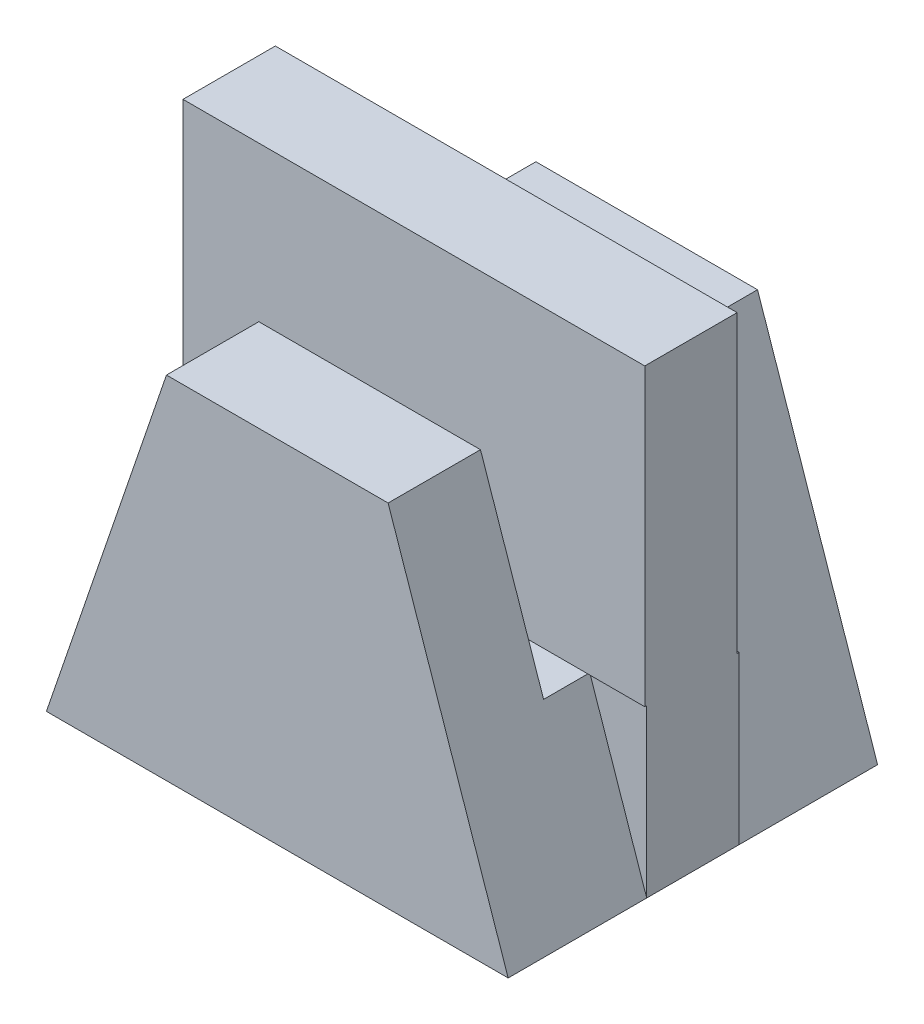
ISO-10303-21;
HEADER;
FILE_DESCRIPTION(('STEP AP214'),'2;1');
FILE_NAME('part.step','',(''),(''),'','','');
FILE_SCHEMA(('AUTOMOTIVE_DESIGN { 1 0 10303 214 1 1 1 1 }'));
ENDSEC;
DATA;
#1=APPLICATION_CONTEXT('core data for automotive mechanical design processes');
#2=APPLICATION_PROTOCOL_DEFINITION('international standard','automotive_design',2000,#1);
#3=PRODUCT_CONTEXT('',#1,'mechanical');
#4=PRODUCT('Part','Part','',(#3));
#5=PRODUCT_RELATED_PRODUCT_CATEGORY('part','',(#4));
#6=PRODUCT_DEFINITION_FORMATION('','',#4);
#7=PRODUCT_DEFINITION_CONTEXT('part definition',#1,'design');
#8=PRODUCT_DEFINITION('design','',#6,#7);
#9=PRODUCT_DEFINITION_SHAPE('','',#8);
#10=(LENGTH_UNIT() NAMED_UNIT(*) SI_UNIT(.MILLI.,.METRE.));
#11=(NAMED_UNIT(*) PLANE_ANGLE_UNIT() SI_UNIT($,.RADIAN.));
#12=(NAMED_UNIT(*) SI_UNIT($,.STERADIAN.) SOLID_ANGLE_UNIT());
#13=UNCERTAINTY_MEASURE_WITH_UNIT(LENGTH_MEASURE(1.E-05),#10,'distance_accuracy_value','');
#14=(GEOMETRIC_REPRESENTATION_CONTEXT(3) GLOBAL_UNCERTAINTY_ASSIGNED_CONTEXT((#13)) GLOBAL_UNIT_ASSIGNED_CONTEXT((#10,
#11,#12)) REPRESENTATION_CONTEXT('',''));
#15=CARTESIAN_POINT('',(0.,0.,0.));
#16=DIRECTION('',(0.,0.,1.));
#17=DIRECTION('',(1.,0.,0.));
#18=AXIS2_PLACEMENT_3D('',#15,#16,#17);
#19=CARTESIAN_POINT('',(25.,0.,40.));
#20=DIRECTION('',(1.,0.,0.));
#21=DIRECTION('',(0.,1.,0.));
#22=AXIS2_PLACEMENT_3D('',#19,#20,#21);
#23=PLANE('',#22);
#24=DIRECTION('',(0.,0.,1.));
#25=VECTOR('',#24,1.);
#26=CARTESIAN_POINT('',(25.,-6.95880702065631,25.));
#27=LINE('',#26,#25);
#28=CARTESIAN_POINT('',(25.,-6.95880702065631,25.));
#29=VERTEX_POINT('',#28);
#30=CARTESIAN_POINT('',(25.,-6.95880702065631,25.211069260478));
#31=VERTEX_POINT('',#30);
#32=EDGE_CURVE('E200',#29,#31,#27,.T.);
#33=ORIENTED_EDGE('',*,*,#32,.F.);
#34=DIRECTION('',(0.,1.,0.));
#35=VECTOR('',#34,1.);
#36=CARTESIAN_POINT('',(25.,-25.,25.));
#37=LINE('',#36,#35);
#38=CARTESIAN_POINT('',(25.,-25.,25.));
#39=VERTEX_POINT('',#38);
#40=EDGE_CURVE('E189',#39,#29,#37,.T.);
#41=ORIENTED_EDGE('',*,*,#40,.F.);
#42=DIRECTION('',(0.,0.,-1.));
#43=VECTOR('',#42,1.);
#44=CARTESIAN_POINT('',(25.,-25.,40.));
#45=LINE('',#44,#43);
#46=CARTESIAN_POINT('',(25.,-25.,15.));
#47=VERTEX_POINT('',#46);
#48=EDGE_CURVE('E183',#39,#47,#45,.T.);
#49=ORIENTED_EDGE('',*,*,#48,.T.);
#50=DIRECTION('',(0.,-1.,0.));
#51=VECTOR('',#50,1.);
#52=CARTESIAN_POINT('',(25.,-6.9588070206563,15.));
#53=LINE('',#52,#51);
#54=CARTESIAN_POINT('',(25.,-6.9588070206563,15.));
#55=VERTEX_POINT('',#54);
#56=EDGE_CURVE('E318',#55,#47,#53,.T.);
#57=ORIENTED_EDGE('',*,*,#56,.F.);
#58=DIRECTION('',(0.,0.,1.));
#59=VECTOR('',#58,1.);
#60=CARTESIAN_POINT('',(25.,-6.9588070206563,0.));
#61=LINE('',#60,#59);
#62=CARTESIAN_POINT('',(25.,-6.9588070206563,15.211069260478));
#63=VERTEX_POINT('',#62);
#64=EDGE_CURVE('E231',#55,#63,#61,.T.);
#65=ORIENTED_EDGE('',*,*,#64,.T.);
#66=DIRECTION('',(0.,1.,0.));
#67=VECTOR('',#66,1.);
#68=CARTESIAN_POINT('',(25.,0.,15.211069260478));
#69=LINE('',#68,#67);
#70=CARTESIAN_POINT('',(25.,25.,15.211069260478));
#71=VERTEX_POINT('',#70);
#72=EDGE_CURVE('E236',#63,#71,#69,.T.);
#73=ORIENTED_EDGE('',*,*,#72,.T.);
#74=DIRECTION('',(0.,0.,-1.));
#75=VECTOR('',#74,1.);
#76=CARTESIAN_POINT('',(25.,25.,40.));
#77=LINE('',#76,#75);
#78=CARTESIAN_POINT('',(25.,25.,25.211069260478));
#79=VERTEX_POINT('',#78);
#80=EDGE_CURVE('E202',#79,#71,#77,.T.);
#81=ORIENTED_EDGE('',*,*,#80,.F.);
#82=DIRECTION('',(0.,-1.,0.));
#83=VECTOR('',#82,1.);
#84=CARTESIAN_POINT('',(25.,0.,25.211069260478));
#85=LINE('',#84,#83);
#86=EDGE_CURVE('E235',#79,#31,#85,.T.);
#87=ORIENTED_EDGE('',*,*,#86,.T.);
#88=EDGE_LOOP('',(#33,#41,#49,#57,#65,#73,#81,#87));
#89=FACE_BOUND('',#88,.T.);
#90=ADVANCED_FACE('F43',(#89),#23,.T.);
#91=CARTESIAN_POINT('',(-25.,0.,40.));
#92=DIRECTION('',(1.,0.,0.));
#93=DIRECTION('',(0.,1.,0.));
#94=AXIS2_PLACEMENT_3D('',#91,#92,#93);
#95=PLANE('',#94);
#96=DIRECTION('',(0.,0.,1.));
#97=VECTOR('',#96,1.);
#98=CARTESIAN_POINT('',(-25.,-6.95880702065631,0.));
#99=LINE('',#98,#97);
#100=CARTESIAN_POINT('',(-25.,-6.95880702065631,15.));
#101=VERTEX_POINT('',#100);
#102=CARTESIAN_POINT('',(-25.,-6.95880702065631,15.211069260478));
#103=VERTEX_POINT('',#102);
#104=EDGE_CURVE('E221',#101,#103,#99,.T.);
#105=ORIENTED_EDGE('',*,*,#104,.F.);
#106=DIRECTION('',(0.,1.,0.));
#107=VECTOR('',#106,1.);
#108=CARTESIAN_POINT('',(-25.,-25.,15.));
#109=LINE('',#108,#107);
#110=CARTESIAN_POINT('',(-25.,-25.,15.));
#111=VERTEX_POINT('',#110);
#112=EDGE_CURVE('E308',#111,#101,#109,.T.);
#113=ORIENTED_EDGE('',*,*,#112,.F.);
#114=DIRECTION('',(0.,0.,-1.));
#115=VECTOR('',#114,1.);
#116=CARTESIAN_POINT('',(-25.,-25.,40.));
#117=LINE('',#116,#115);
#118=CARTESIAN_POINT('',(-25.,-25.,25.));
#119=VERTEX_POINT('',#118);
#120=EDGE_CURVE('E212',#119,#111,#117,.T.);
#121=ORIENTED_EDGE('',*,*,#120,.F.);
#122=DIRECTION('',(0.,-1.,0.));
#123=VECTOR('',#122,1.);
#124=CARTESIAN_POINT('',(-25.,-25.,25.));
#125=LINE('',#124,#123);
#126=CARTESIAN_POINT('',(-25.,-6.95880702065632,25.));
#127=VERTEX_POINT('',#126);
#128=EDGE_CURVE('E295',#127,#119,#125,.T.);
#129=ORIENTED_EDGE('',*,*,#128,.F.);
#130=DIRECTION('',(0.,0.,1.));
#131=VECTOR('',#130,1.);
#132=CARTESIAN_POINT('',(-25.,-6.95880702065632,25.));
#133=LINE('',#132,#131);
#134=CARTESIAN_POINT('',(-25.,-6.95880702065632,25.211069260478));
#135=VERTEX_POINT('',#134);
#136=EDGE_CURVE('E286',#127,#135,#133,.T.);
#137=ORIENTED_EDGE('',*,*,#136,.T.);
#138=DIRECTION('',(0.,-1.,0.));
#139=VECTOR('',#138,1.);
#140=CARTESIAN_POINT('',(-25.,0.,25.211069260478));
#141=LINE('',#140,#139);
#142=CARTESIAN_POINT('',(-25.,25.,25.211069260478));
#143=VERTEX_POINT('',#142);
#144=EDGE_CURVE('E246',#143,#135,#141,.T.);
#145=ORIENTED_EDGE('',*,*,#144,.F.);
#146=DIRECTION('',(0.,0.,-1.));
#147=VECTOR('',#146,1.);
#148=CARTESIAN_POINT('',(-25.,25.,40.));
#149=LINE('',#148,#147);
#150=CARTESIAN_POINT('',(-25.,25.,15.211069260478));
#151=VERTEX_POINT('',#150);
#152=EDGE_CURVE('E203',#143,#151,#149,.T.);
#153=ORIENTED_EDGE('',*,*,#152,.T.);
#154=DIRECTION('',(0.,1.,0.));
#155=VECTOR('',#154,1.);
#156=CARTESIAN_POINT('',(-25.,0.,15.211069260478));
#157=LINE('',#156,#155);
#158=EDGE_CURVE('E232',#103,#151,#157,.T.);
#159=ORIENTED_EDGE('',*,*,#158,.F.);
#160=EDGE_LOOP('',(#105,#113,#121,#129,#137,#145,#153,#159));
#161=FACE_BOUND('',#160,.T.);
#162=ADVANCED_FACE('F341',(#161),#95,.F.);
#163=CARTESIAN_POINT('',(0.,25.,40.));
#164=DIRECTION('',(0.,1.,0.));
#165=DIRECTION('',(-1.,0.,0.));
#166=AXIS2_PLACEMENT_3D('',#163,#164,#165);
#167=PLANE('',#166);
#168=ORIENTED_EDGE('',*,*,#152,.F.);
#169=DIRECTION('',(1.,0.,0.));
#170=VECTOR('',#169,1.);
#171=CARTESIAN_POINT('',(-25.,25.,25.211069260478));
#172=LINE('',#171,#170);
#173=EDGE_CURVE('E254',#143,#79,#172,.T.);
#174=ORIENTED_EDGE('',*,*,#173,.T.);
#175=ORIENTED_EDGE('',*,*,#80,.T.);
#176=DIRECTION('',(1.,0.,0.));
#177=VECTOR('',#176,1.);
#178=CARTESIAN_POINT('',(-25.,25.,15.211069260478));
#179=LINE('',#178,#177);
#180=EDGE_CURVE('E223',#151,#71,#179,.T.);
#181=ORIENTED_EDGE('',*,*,#180,.F.);
#182=EDGE_LOOP('',(#168,#174,#175,#181));
#183=FACE_BOUND('',#182,.T.);
#184=ADVANCED_FACE('F395',(#183),#167,.T.);
#185=CARTESIAN_POINT('',(0.,0.,40.));
#186=DIRECTION('',(0.,0.,1.));
#187=DIRECTION('',(1.,0.,0.));
#188=AXIS2_PLACEMENT_3D('',#185,#186,#187);
#189=PLANE('',#188);
#190=DIRECTION('',(0.323373843640664,-0.94627129156974,0.));
#191=VECTOR('',#190,1.);
#192=CARTESIAN_POINT('',(12.,13.0411929793437,40.));
#193=LINE('',#192,#191);
#194=CARTESIAN_POINT('',(12.,13.0411929793437,40.));
#195=VERTEX_POINT('',#194);
#196=CARTESIAN_POINT('',(25.,-25.,40.));
#197=VERTEX_POINT('',#196);
#198=EDGE_CURVE('E177',#195,#197,#193,.T.);
#199=ORIENTED_EDGE('',*,*,#198,.F.);
#200=DIRECTION('',(1.,0.,0.));
#201=VECTOR('',#200,1.);
#202=CARTESIAN_POINT('',(-25.,13.0411929793437,40.));
#203=LINE('',#202,#201);
#204=CARTESIAN_POINT('',(-12.,13.0411929793437,40.));
#205=VERTEX_POINT('',#204);
#206=EDGE_CURVE('E213',#205,#195,#203,.T.);
#207=ORIENTED_EDGE('',*,*,#206,.F.);
#208=DIRECTION('',(0.323373843640664,0.94627129156974,0.));
#209=VECTOR('',#208,1.);
#210=CARTESIAN_POINT('',(-25.,-25.,40.));
#211=LINE('',#210,#209);
#212=CARTESIAN_POINT('',(-25.,-25.,40.));
#213=VERTEX_POINT('',#212);
#214=EDGE_CURVE('E284',#213,#205,#211,.T.);
#215=ORIENTED_EDGE('',*,*,#214,.F.);
#216=DIRECTION('',(1.,0.,0.));
#217=VECTOR('',#216,1.);
#218=CARTESIAN_POINT('',(0.,-25.,40.));
#219=LINE('',#218,#217);
#220=EDGE_CURVE('E211',#213,#197,#219,.T.);
#221=ORIENTED_EDGE('',*,*,#220,.T.);
#222=EDGE_LOOP('',(#199,#207,#215,#221));
#223=FACE_BOUND('',#222,.T.);
#224=ADVANCED_FACE('F365',(#223),#189,.T.);
#225=CARTESIAN_POINT('',(0.,0.,0.));
#226=DIRECTION('',(0.,0.,1.));
#227=DIRECTION('',(1.,0.,0.));
#228=AXIS2_PLACEMENT_3D('',#225,#226,#227);
#229=PLANE('',#228);
#230=DIRECTION('',(1.,0.,0.));
#231=VECTOR('',#230,1.);
#232=CARTESIAN_POINT('',(0.,-25.,0.));
#233=LINE('',#232,#231);
#234=CARTESIAN_POINT('',(-25.,-25.,0.));
#235=VERTEX_POINT('',#234);
#236=CARTESIAN_POINT('',(25.,-25.,0.));
#237=VERTEX_POINT('',#236);
#238=EDGE_CURVE('E215',#235,#237,#233,.T.);
#239=ORIENTED_EDGE('',*,*,#238,.F.);
#240=DIRECTION('',(-0.323373843640664,-0.94627129156974,0.));
#241=VECTOR('',#240,1.);
#242=CARTESIAN_POINT('',(-12.,13.0411929793437,0.));
#243=LINE('',#242,#241);
#244=CARTESIAN_POINT('',(-12.,13.0411929793437,0.));
#245=VERTEX_POINT('',#244);
#246=EDGE_CURVE('E270',#245,#235,#243,.T.);
#247=ORIENTED_EDGE('',*,*,#246,.F.);
#248=DIRECTION('',(1.,0.,0.));
#249=VECTOR('',#248,1.);
#250=CARTESIAN_POINT('',(-25.,13.0411929793437,0.));
#251=LINE('',#250,#249);
#252=CARTESIAN_POINT('',(12.,13.0411929793437,0.));
#253=VERTEX_POINT('',#252);
#254=EDGE_CURVE('E217',#245,#253,#251,.T.);
#255=ORIENTED_EDGE('',*,*,#254,.T.);
#256=DIRECTION('',(-0.323373843640664,0.94627129156974,0.));
#257=VECTOR('',#256,1.);
#258=CARTESIAN_POINT('',(12.,13.0411929793437,0.));
#259=LINE('',#258,#257);
#260=EDGE_CURVE('E271',#237,#253,#259,.T.);
#261=ORIENTED_EDGE('',*,*,#260,.F.);
#262=EDGE_LOOP('',(#239,#247,#255,#261));
#263=FACE_BOUND('',#262,.T.);
#264=ADVANCED_FACE('F368',(#263),#229,.F.);
#265=CARTESIAN_POINT('',(0.,-25.,40.));
#266=DIRECTION('',(0.,1.,0.));
#267=DIRECTION('',(0.,0.,1.));
#268=AXIS2_PLACEMENT_3D('',#265,#266,#267);
#269=PLANE('',#268);
#270=ORIENTED_EDGE('',*,*,#238,.T.);
#271=DIRECTION('',(0.,0.,-1.));
#272=VECTOR('',#271,1.);
#273=CARTESIAN_POINT('',(25.,-25.,10.));
#274=LINE('',#273,#272);
#275=EDGE_CURVE('E197',#47,#237,#274,.T.);
#276=ORIENTED_EDGE('',*,*,#275,.F.);
#277=ORIENTED_EDGE('',*,*,#48,.F.);
#278=EDGE_CURVE('E51',#197,#39,#45,.T.);
#279=ORIENTED_EDGE('',*,*,#278,.F.);
#280=ORIENTED_EDGE('',*,*,#220,.F.);
#281=EDGE_CURVE('E209',#213,#119,#117,.T.);
#282=ORIENTED_EDGE('',*,*,#281,.T.);
#283=ORIENTED_EDGE('',*,*,#120,.T.);
#284=DIRECTION('',(0.,0.,-1.));
#285=VECTOR('',#284,1.);
#286=CARTESIAN_POINT('',(-25.,-25.,10.));
#287=LINE('',#286,#285);
#288=EDGE_CURVE('E237',#111,#235,#287,.T.);
#289=ORIENTED_EDGE('',*,*,#288,.T.);
#290=EDGE_LOOP('',(#270,#276,#277,#279,#280,#282,#283,#289));
#291=FACE_BOUND('',#290,.T.);
#292=ADVANCED_FACE('F44',(#291),#269,.F.);
#293=CARTESIAN_POINT('',(-25.,0.,10.));
#294=DIRECTION('',(0.,0.,1.));
#295=DIRECTION('',(0.,-1.,0.));
#296=AXIS2_PLACEMENT_3D('',#293,#294,#295);
#297=PLANE('',#296);
#298=DIRECTION('',(-0.323373843640664,-0.94627129156974,0.));
#299=VECTOR('',#298,1.);
#300=CARTESIAN_POINT('',(-12.,13.0411929793437,10.));
#301=LINE('',#300,#299);
#302=CARTESIAN_POINT('',(-12.,13.0411929793437,10.));
#303=VERTEX_POINT('',#302);
#304=CARTESIAN_POINT('',(-18.8346962762493,-6.95880702065632,10.));
#305=VERTEX_POINT('',#304);
#306=EDGE_CURVE('E261',#303,#305,#301,.T.);
#307=ORIENTED_EDGE('',*,*,#306,.T.);
#308=DIRECTION('',(1.,0.,0.));
#309=VECTOR('',#308,1.);
#310=CARTESIAN_POINT('',(-25.,-6.95880702065631,10.));
#311=LINE('',#310,#309);
#312=CARTESIAN_POINT('',(18.8346962762493,-6.9588070206563,10.));
#313=VERTEX_POINT('',#312);
#314=EDGE_CURVE('E230',#305,#313,#311,.T.);
#315=ORIENTED_EDGE('',*,*,#314,.T.);
#316=DIRECTION('',(-0.323373843640664,0.94627129156974,0.));
#317=VECTOR('',#316,1.);
#318=CARTESIAN_POINT('',(12.,13.0411929793437,10.));
#319=LINE('',#318,#317);
#320=CARTESIAN_POINT('',(12.,13.0411929793437,10.));
#321=VERTEX_POINT('',#320);
#322=EDGE_CURVE('E275',#313,#321,#319,.T.);
#323=ORIENTED_EDGE('',*,*,#322,.T.);
#324=DIRECTION('',(1.,0.,0.));
#325=VECTOR('',#324,1.);
#326=CARTESIAN_POINT('',(-25.,13.0411929793437,10.));
#327=LINE('',#326,#325);
#328=EDGE_CURVE('E220',#303,#321,#327,.T.);
#329=ORIENTED_EDGE('',*,*,#328,.F.);
#330=EDGE_LOOP('',(#307,#315,#323,#329));
#331=FACE_BOUND('',#330,.T.);
#332=ADVANCED_FACE('F377',(#331),#297,.T.);
#333=CARTESIAN_POINT('',(-25.,-6.95880702065631,0.));
#334=DIRECTION('',(0.,1.,0.));
#335=DIRECTION('',(-1.,0.,0.));
#336=AXIS2_PLACEMENT_3D('',#333,#334,#335);
#337=PLANE('',#336);
#338=DIRECTION('',(0.,0.,-1.));
#339=VECTOR('',#338,1.);
#340=CARTESIAN_POINT('',(18.8346962762493,-6.9588070206563,15.));
#341=LINE('',#340,#339);
#342=CARTESIAN_POINT('',(18.8346962762493,-6.9588070206563,15.));
#343=VERTEX_POINT('',#342);
#344=EDGE_CURVE('E312',#343,#313,#341,.T.);
#345=ORIENTED_EDGE('',*,*,#344,.T.);
#346=ORIENTED_EDGE('',*,*,#314,.F.);
#347=DIRECTION('',(0.,0.,-1.));
#348=VECTOR('',#347,1.);
#349=CARTESIAN_POINT('',(-18.8346962762493,-6.95880702065631,15.));
#350=LINE('',#349,#348);
#351=CARTESIAN_POINT('',(-18.8346962762493,-6.95880702065631,15.));
#352=VERTEX_POINT('',#351);
#353=EDGE_CURVE('E303',#352,#305,#350,.T.);
#354=ORIENTED_EDGE('',*,*,#353,.F.);
#355=DIRECTION('',(1.,0.,0.));
#356=VECTOR('',#355,1.);
#357=CARTESIAN_POINT('',(-25.,-6.95880702065631,15.));
#358=LINE('',#357,#356);
#359=EDGE_CURVE('E304',#101,#352,#358,.T.);
#360=ORIENTED_EDGE('',*,*,#359,.F.);
#361=ORIENTED_EDGE('',*,*,#104,.T.);
#362=DIRECTION('',(1.,0.,0.));
#363=VECTOR('',#362,1.);
#364=CARTESIAN_POINT('',(-25.,-6.95880702065631,15.211069260478));
#365=LINE('',#364,#363);
#366=EDGE_CURVE('E228',#103,#63,#365,.T.);
#367=ORIENTED_EDGE('',*,*,#366,.T.);
#368=ORIENTED_EDGE('',*,*,#64,.F.);
#369=DIRECTION('',(1.,0.,0.));
#370=VECTOR('',#369,1.);
#371=CARTESIAN_POINT('',(18.8346962762493,-6.9588070206563,15.));
#372=LINE('',#371,#370);
#373=EDGE_CURVE('E314',#343,#55,#372,.T.);
#374=ORIENTED_EDGE('',*,*,#373,.F.);
#375=EDGE_LOOP('',(#345,#346,#354,#360,#361,#367,#368,#374));
#376=FACE_BOUND('',#375,.T.);
#377=ADVANCED_FACE('F383',(#376),#337,.T.);
#378=CARTESIAN_POINT('',(-25.,0.,15.211069260478));
#379=DIRECTION('',(0.,0.,-1.));
#380=DIRECTION('',(0.,1.,0.));
#381=AXIS2_PLACEMENT_3D('',#378,#379,#380);
#382=PLANE('',#381);
#383=ORIENTED_EDGE('',*,*,#72,.F.);
#384=ORIENTED_EDGE('',*,*,#366,.F.);
#385=ORIENTED_EDGE('',*,*,#158,.T.);
#386=ORIENTED_EDGE('',*,*,#180,.T.);
#387=EDGE_LOOP('',(#383,#384,#385,#386));
#388=FACE_BOUND('',#387,.T.);
#389=ADVANCED_FACE('F394',(#388),#382,.T.);
#390=CARTESIAN_POINT('',(-25.,13.0411929793437,0.));
#391=DIRECTION('',(0.,1.,0.));
#392=DIRECTION('',(0.,0.,1.));
#393=AXIS2_PLACEMENT_3D('',#390,#391,#392);
#394=PLANE('',#393);
#395=DIRECTION('',(0.,0.,-1.));
#396=VECTOR('',#395,1.);
#397=CARTESIAN_POINT('',(-12.,13.0411929793437,10.));
#398=LINE('',#397,#396);
#399=EDGE_CURVE('E266',#303,#245,#398,.T.);
#400=ORIENTED_EDGE('',*,*,#399,.F.);
#401=ORIENTED_EDGE('',*,*,#328,.T.);
#402=DIRECTION('',(0.,0.,-1.));
#403=VECTOR('',#402,1.);
#404=CARTESIAN_POINT('',(12.,13.0411929793437,10.));
#405=LINE('',#404,#403);
#406=EDGE_CURVE('E265',#321,#253,#405,.T.);
#407=ORIENTED_EDGE('',*,*,#406,.T.);
#408=ORIENTED_EDGE('',*,*,#254,.F.);
#409=EDGE_LOOP('',(#400,#401,#407,#408));
#410=FACE_BOUND('',#409,.T.);
#411=ADVANCED_FACE('F374',(#410),#394,.T.);
#412=CARTESIAN_POINT('',(-25.,13.0411929793437,0.));
#413=DIRECTION('',(0.,1.,0.));
#414=DIRECTION('',(-1.,0.,0.));
#415=AXIS2_PLACEMENT_3D('',#412,#413,#414);
#416=PLANE('',#415);
#417=DIRECTION('',(0.,0.,1.));
#418=VECTOR('',#417,1.);
#419=CARTESIAN_POINT('',(12.,13.0411929793437,30.));
#420=LINE('',#419,#418);
#421=CARTESIAN_POINT('',(12.,13.0411929793437,30.));
#422=VERTEX_POINT('',#421);
#423=EDGE_CURVE('E273',#422,#195,#420,.T.);
#424=ORIENTED_EDGE('',*,*,#423,.F.);
#425=DIRECTION('',(1.,0.,0.));
#426=VECTOR('',#425,1.);
#427=CARTESIAN_POINT('',(-25.,13.0411929793437,30.));
#428=LINE('',#427,#426);
#429=CARTESIAN_POINT('',(-12.,13.0411929793437,30.));
#430=VERTEX_POINT('',#429);
#431=EDGE_CURVE('E245',#430,#422,#428,.T.);
#432=ORIENTED_EDGE('',*,*,#431,.F.);
#433=DIRECTION('',(0.,0.,1.));
#434=VECTOR('',#433,1.);
#435=CARTESIAN_POINT('',(-12.,13.0411929793437,30.));
#436=LINE('',#435,#434);
#437=EDGE_CURVE('E60',#430,#205,#436,.T.);
#438=ORIENTED_EDGE('',*,*,#437,.T.);
#439=ORIENTED_EDGE('',*,*,#206,.T.);
#440=EDGE_LOOP('',(#424,#432,#438,#439));
#441=FACE_BOUND('',#440,.T.);
#442=ADVANCED_FACE('F360',(#441),#416,.T.);
#443=CARTESIAN_POINT('',(-25.,0.,25.211069260478));
#444=DIRECTION('',(0.,0.,1.));
#445=DIRECTION('',(1.,0.,0.));
#446=AXIS2_PLACEMENT_3D('',#443,#444,#445);
#447=PLANE('',#446);
#448=ORIENTED_EDGE('',*,*,#86,.F.);
#449=ORIENTED_EDGE('',*,*,#173,.F.);
#450=ORIENTED_EDGE('',*,*,#144,.T.);
#451=DIRECTION('',(1.,0.,0.));
#452=VECTOR('',#451,1.);
#453=CARTESIAN_POINT('',(-25.,-6.95880702065631,25.211069260478));
#454=LINE('',#453,#452);
#455=CARTESIAN_POINT('',(-18.8346962762493,-6.95880702065631,25.211069260478));
#456=VERTEX_POINT('',#455);
#457=EDGE_CURVE('E249',#135,#456,#454,.T.);
#458=ORIENTED_EDGE('',*,*,#457,.T.);
#459=CARTESIAN_POINT('',(18.8346962762493,-6.95880702065631,25.211069260478));
#460=VERTEX_POINT('',#459);
#461=EDGE_CURVE('E248',#456,#460,#454,.T.);
#462=ORIENTED_EDGE('',*,*,#461,.T.);
#463=DIRECTION('',(-1.,0.,0.));
#464=VECTOR('',#463,1.);
#465=CARTESIAN_POINT('',(-25.,-6.95880702065627,25.211069260478));
#466=LINE('',#465,#464);
#467=EDGE_CURVE('E324',#31,#460,#466,.T.);
#468=ORIENTED_EDGE('',*,*,#467,.F.);
#469=EDGE_LOOP('',(#448,#449,#450,#458,#462,#468));
#470=FACE_BOUND('',#469,.T.);
#471=ADVANCED_FACE('F337',(#470),#447,.T.);
#472=CARTESIAN_POINT('',(-25.,-6.95880702065631,0.));
#473=DIRECTION('',(0.,1.,0.));
#474=DIRECTION('',(-1.,0.,0.));
#475=AXIS2_PLACEMENT_3D('',#472,#473,#474);
#476=PLANE('',#475);
#477=DIRECTION('',(0.,0.,1.));
#478=VECTOR('',#477,1.);
#479=CARTESIAN_POINT('',(18.8346962762493,-6.95880702065631,25.));
#480=LINE('',#479,#478);
#481=CARTESIAN_POINT('',(18.8346962762493,-6.95880702065631,30.));
#482=VERTEX_POINT('',#481);
#483=EDGE_CURVE('E63',#460,#482,#480,.T.);
#484=ORIENTED_EDGE('',*,*,#483,.F.);
#485=ORIENTED_EDGE('',*,*,#461,.F.);
#486=DIRECTION('',(0.,0.,1.));
#487=VECTOR('',#486,1.);
#488=CARTESIAN_POINT('',(-18.8346962762493,-6.95880702065631,25.));
#489=LINE('',#488,#487);
#490=CARTESIAN_POINT('',(-18.8346962762493,-6.95880702065631,30.));
#491=VERTEX_POINT('',#490);
#492=EDGE_CURVE('E293',#456,#491,#489,.T.);
#493=ORIENTED_EDGE('',*,*,#492,.T.);
#494=DIRECTION('',(1.,0.,0.));
#495=VECTOR('',#494,1.);
#496=CARTESIAN_POINT('',(-25.,-6.95880702065632,30.));
#497=LINE('',#496,#495);
#498=EDGE_CURVE('E244',#491,#482,#497,.T.);
#499=ORIENTED_EDGE('',*,*,#498,.T.);
#500=EDGE_LOOP('',(#484,#485,#493,#499));
#501=FACE_BOUND('',#500,.T.);
#502=ADVANCED_FACE('F332',(#501),#476,.T.);
#503=CARTESIAN_POINT('',(-25.,0.,30.));
#504=DIRECTION('',(0.,0.,-1.));
#505=DIRECTION('',(-1.,0.,0.));
#506=AXIS2_PLACEMENT_3D('',#503,#504,#505);
#507=PLANE('',#506);
#508=DIRECTION('',(0.323373843640664,-0.94627129156974,0.));
#509=VECTOR('',#508,1.);
#510=CARTESIAN_POINT('',(12.,13.0411929793437,30.));
#511=LINE('',#510,#509);
#512=EDGE_CURVE('E283',#422,#482,#511,.T.);
#513=ORIENTED_EDGE('',*,*,#512,.T.);
#514=ORIENTED_EDGE('',*,*,#498,.F.);
#515=DIRECTION('',(-0.323373843640664,-0.94627129156974,0.));
#516=VECTOR('',#515,1.);
#517=CARTESIAN_POINT('',(-17.350015382957,-2.61426606877343,30.));
#518=LINE('',#517,#516);
#519=EDGE_CURVE('E11',#430,#491,#518,.T.);
#520=ORIENTED_EDGE('',*,*,#519,.F.);
#521=ORIENTED_EDGE('',*,*,#431,.T.);
#522=EDGE_LOOP('',(#513,#514,#520,#521));
#523=FACE_BOUND('',#522,.T.);
#524=ADVANCED_FACE('F358',(#523),#507,.T.);
#525=CARTESIAN_POINT('',(12.,13.0411929793437,10.));
#526=DIRECTION('',(-0.94627129156974,-0.323373843640664,0.));
#527=DIRECTION('',(0.323373843640664,-0.94627129156974,0.));
#528=AXIS2_PLACEMENT_3D('',#525,#526,#527);
#529=PLANE('',#528);
#530=ORIENTED_EDGE('',*,*,#260,.T.);
#531=ORIENTED_EDGE('',*,*,#406,.F.);
#532=ORIENTED_EDGE('',*,*,#322,.F.);
#533=ORIENTED_EDGE('',*,*,#344,.F.);
#534=DIRECTION('',(-0.323373843640664,0.94627129156974,0.));
#535=VECTOR('',#534,1.);
#536=CARTESIAN_POINT('',(25.,-25.,15.));
#537=LINE('',#536,#535);
#538=EDGE_CURVE('E320',#47,#343,#537,.T.);
#539=ORIENTED_EDGE('',*,*,#538,.F.);
#540=ORIENTED_EDGE('',*,*,#275,.T.);
#541=EDGE_LOOP('',(#530,#531,#532,#533,#539,#540));
#542=FACE_BOUND('',#541,.T.);
#543=ADVANCED_FACE('F371',(#542),#529,.F.);
#544=CARTESIAN_POINT('',(-12.,13.0411929793437,10.));
#545=DIRECTION('',(0.94627129156974,-0.323373843640664,0.));
#546=DIRECTION('',(0.323373843640664,0.94627129156974,0.));
#547=AXIS2_PLACEMENT_3D('',#544,#545,#546);
#548=PLANE('',#547);
#549=ORIENTED_EDGE('',*,*,#246,.T.);
#550=ORIENTED_EDGE('',*,*,#288,.F.);
#551=DIRECTION('',(-0.323373843640664,-0.94627129156974,0.));
#552=VECTOR('',#551,1.);
#553=CARTESIAN_POINT('',(-18.8346962762493,-6.95880702065631,15.));
#554=LINE('',#553,#552);
#555=EDGE_CURVE('E309',#352,#111,#554,.T.);
#556=ORIENTED_EDGE('',*,*,#555,.F.);
#557=ORIENTED_EDGE('',*,*,#353,.T.);
#558=ORIENTED_EDGE('',*,*,#306,.F.);
#559=ORIENTED_EDGE('',*,*,#399,.T.);
#560=EDGE_LOOP('',(#549,#550,#556,#557,#558,#559));
#561=FACE_BOUND('',#560,.T.);
#562=ADVANCED_FACE('F511',(#561),#548,.F.);
#563=CARTESIAN_POINT('',(-25.,-25.,30.));
#564=DIRECTION('',(0.94627129156974,-0.323373843640664,0.));
#565=DIRECTION('',(0.323373843640664,0.94627129156974,0.));
#566=AXIS2_PLACEMENT_3D('',#563,#564,#565);
#567=PLANE('',#566);
#568=ORIENTED_EDGE('',*,*,#214,.T.);
#569=ORIENTED_EDGE('',*,*,#437,.F.);
#570=ORIENTED_EDGE('',*,*,#519,.T.);
#571=ORIENTED_EDGE('',*,*,#492,.F.);
#572=CARTESIAN_POINT('',(-18.8346962762493,-6.95880702065631,25.));
#573=VERTEX_POINT('',#572);
#574=EDGE_CURVE('E289',#573,#456,#489,.T.);
#575=ORIENTED_EDGE('',*,*,#574,.F.);
#576=DIRECTION('',(0.323373843640664,0.94627129156974,0.));
#577=VECTOR('',#576,1.);
#578=CARTESIAN_POINT('',(-18.8346962762493,-6.95880702065631,25.));
#579=LINE('',#578,#577);
#580=EDGE_CURVE('E297',#119,#573,#579,.T.);
#581=ORIENTED_EDGE('',*,*,#580,.F.);
#582=ORIENTED_EDGE('',*,*,#281,.F.);
#583=EDGE_LOOP('',(#568,#569,#570,#571,#575,#581,#582));
#584=FACE_BOUND('',#583,.T.);
#585=ADVANCED_FACE('F352',(#584),#567,.F.);
#586=CARTESIAN_POINT('',(12.,13.0411929793437,30.));
#587=DIRECTION('',(-0.94627129156974,-0.323373843640664,0.));
#588=DIRECTION('',(0.323373843640664,-0.94627129156974,0.));
#589=AXIS2_PLACEMENT_3D('',#586,#587,#588);
#590=PLANE('',#589);
#591=ORIENTED_EDGE('',*,*,#198,.T.);
#592=ORIENTED_EDGE('',*,*,#278,.T.);
#593=DIRECTION('',(0.323373843640664,-0.94627129156974,0.));
#594=VECTOR('',#593,1.);
#595=CARTESIAN_POINT('',(18.8346962762493,-6.95880702065631,25.));
#596=LINE('',#595,#594);
#597=CARTESIAN_POINT('',(18.8346962762493,-6.95880702065631,25.));
#598=VERTEX_POINT('',#597);
#599=EDGE_CURVE('E176',#598,#39,#596,.T.);
#600=ORIENTED_EDGE('',*,*,#599,.F.);
#601=EDGE_CURVE('E323',#598,#460,#480,.T.);
#602=ORIENTED_EDGE('',*,*,#601,.T.);
#603=ORIENTED_EDGE('',*,*,#483,.T.);
#604=ORIENTED_EDGE('',*,*,#512,.F.);
#605=ORIENTED_EDGE('',*,*,#423,.T.);
#606=EDGE_LOOP('',(#591,#592,#600,#602,#603,#604,#605));
#607=FACE_BOUND('',#606,.T.);
#608=ADVANCED_FACE('F174',(#607),#590,.F.);
#609=CARTESIAN_POINT('',(-25.,-6.95880702065632,25.));
#610=DIRECTION('',(0.,1.,0.));
#611=DIRECTION('',(-1.,0.,0.));
#612=AXIS2_PLACEMENT_3D('',#609,#610,#611);
#613=PLANE('',#612);
#614=ORIENTED_EDGE('',*,*,#457,.F.);
#615=ORIENTED_EDGE('',*,*,#136,.F.);
#616=DIRECTION('',(-1.,0.,0.));
#617=VECTOR('',#616,1.);
#618=CARTESIAN_POINT('',(-25.,-6.95880702065632,25.));
#619=LINE('',#618,#617);
#620=EDGE_CURVE('E300',#573,#127,#619,.T.);
#621=ORIENTED_EDGE('',*,*,#620,.F.);
#622=ORIENTED_EDGE('',*,*,#574,.T.);
#623=EDGE_LOOP('',(#614,#615,#621,#622));
#624=FACE_BOUND('',#623,.T.);
#625=ADVANCED_FACE('F339',(#624),#613,.F.);
#626=CARTESIAN_POINT('',(0.,0.,25.));
#627=DIRECTION('',(0.,0.,1.));
#628=DIRECTION('',(1.,0.,0.));
#629=AXIS2_PLACEMENT_3D('',#626,#627,#628);
#630=PLANE('',#629);
#631=ORIENTED_EDGE('',*,*,#580,.T.);
#632=ORIENTED_EDGE('',*,*,#620,.T.);
#633=ORIENTED_EDGE('',*,*,#128,.T.);
#634=EDGE_LOOP('',(#631,#632,#633));
#635=FACE_BOUND('',#634,.T.);
#636=ADVANCED_FACE('F347',(#635),#630,.T.);
#637=CARTESIAN_POINT('',(0.,0.,15.));
#638=DIRECTION('',(0.,0.,1.));
#639=DIRECTION('',(1.,0.,0.));
#640=AXIS2_PLACEMENT_3D('',#637,#638,#639);
#641=PLANE('',#640);
#642=ORIENTED_EDGE('',*,*,#555,.T.);
#643=ORIENTED_EDGE('',*,*,#112,.T.);
#644=ORIENTED_EDGE('',*,*,#359,.T.);
#645=EDGE_LOOP('',(#642,#643,#644));
#646=FACE_BOUND('',#645,.T.);
#647=ADVANCED_FACE('F476',(#646),#641,.F.);
#648=CARTESIAN_POINT('',(0.,0.,15.));
#649=DIRECTION('',(0.,0.,1.));
#650=DIRECTION('',(1.,0.,0.));
#651=AXIS2_PLACEMENT_3D('',#648,#649,#650);
#652=PLANE('',#651);
#653=ORIENTED_EDGE('',*,*,#56,.T.);
#654=ORIENTED_EDGE('',*,*,#538,.T.);
#655=ORIENTED_EDGE('',*,*,#373,.T.);
#656=EDGE_LOOP('',(#653,#654,#655));
#657=FACE_BOUND('',#656,.T.);
#658=ADVANCED_FACE('F384',(#657),#652,.F.);
#659=CARTESIAN_POINT('',(25.,-6.95880702065631,25.));
#660=DIRECTION('',(0.,1.,0.));
#661=DIRECTION('',(-1.,0.,0.));
#662=AXIS2_PLACEMENT_3D('',#659,#660,#661);
#663=PLANE('',#662);
#664=ORIENTED_EDGE('',*,*,#467,.T.);
#665=ORIENTED_EDGE('',*,*,#601,.F.);
#666=DIRECTION('',(-1.,0.,0.));
#667=VECTOR('',#666,1.);
#668=CARTESIAN_POINT('',(25.,-6.95880702065631,25.));
#669=LINE('',#668,#667);
#670=EDGE_CURVE('E188',#29,#598,#669,.T.);
#671=ORIENTED_EDGE('',*,*,#670,.F.);
#672=ORIENTED_EDGE('',*,*,#32,.T.);
#673=EDGE_LOOP('',(#664,#665,#671,#672));
#674=FACE_BOUND('',#673,.T.);
#675=ADVANCED_FACE('F457',(#674),#663,.F.);
#676=CARTESIAN_POINT('',(0.,0.,25.));
#677=DIRECTION('',(0.,0.,-1.));
#678=DIRECTION('',(-1.,0.,0.));
#679=AXIS2_PLACEMENT_3D('',#676,#677,#678);
#680=PLANE('',#679);
#681=ORIENTED_EDGE('',*,*,#599,.T.);
#682=ORIENTED_EDGE('',*,*,#40,.T.);
#683=ORIENTED_EDGE('',*,*,#670,.T.);
#684=EDGE_LOOP('',(#681,#682,#683));
#685=FACE_BOUND('',#684,.T.);
#686=ADVANCED_FACE('F190',(#685),#680,.F.);
#687=CLOSED_SHELL('',(#90,#162,#184,#224,#264,#292,#332,#377,#389,#411,#442,#471,#502,#524,#543,
#562,#585,#608,#625,#636,#647,#658,#675,#686));
#688=MANIFOLD_SOLID_BREP('B2',#687);
#689=ADVANCED_BREP_SHAPE_REPRESENTATION('',(#18,#688),#14);
#690=SHAPE_DEFINITION_REPRESENTATION(#9,#689);
ENDSEC;
END-ISO-10303-21;
